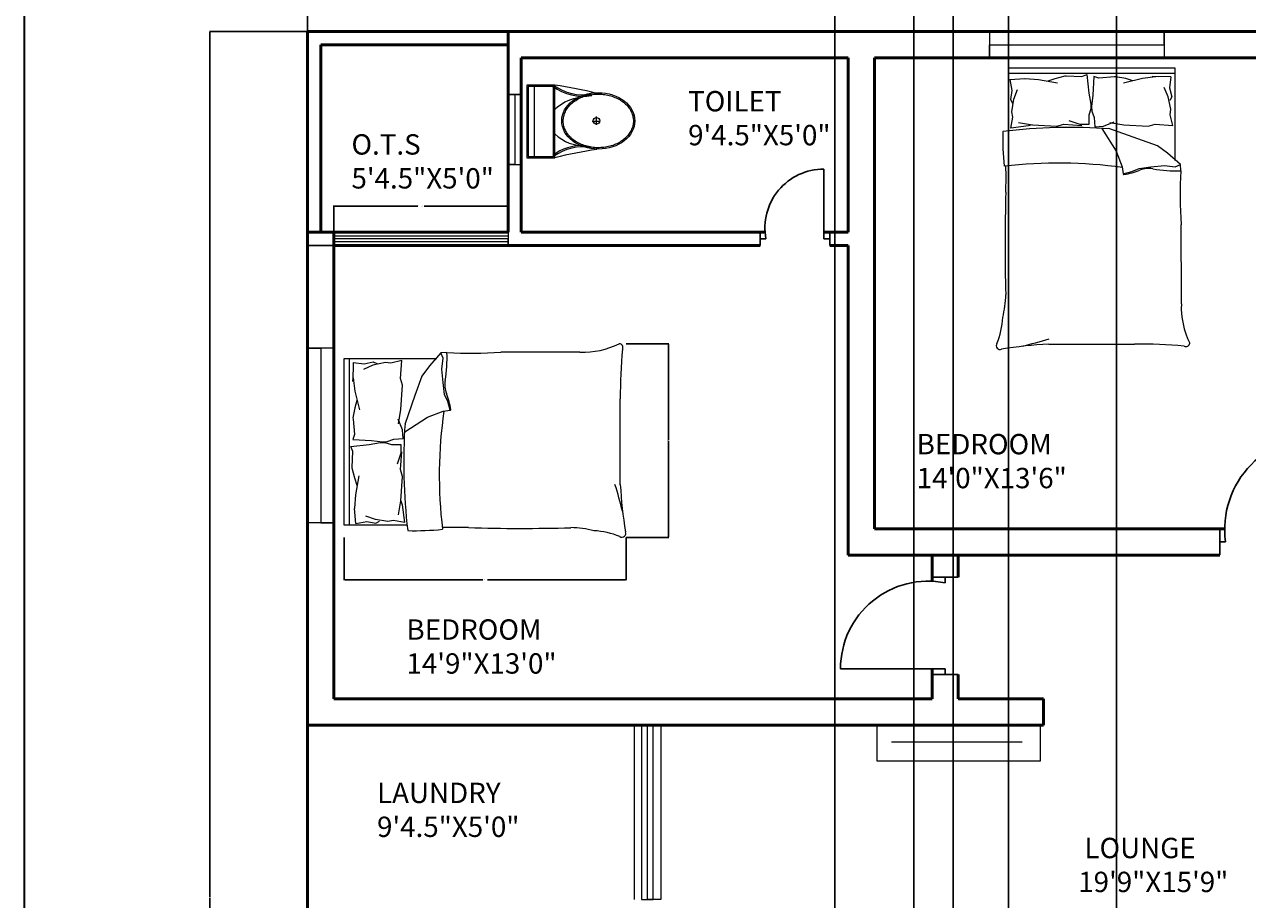
# Model space of a CAD drawing. Units: inches. Extents: x 2215 to 3724, y 1009 to 2124.
# Tile 4 of 11: x 2215 to 2636, y 1449 to 1750. Entities that reach past the tile are written whole.
import ezdxf

# ---------------------------------------------------------------- set-up
doc = ezdxf.new("R2010")
doc.units = ezdxf.units.IN
for name, color, linetype, lineweight in [('A-ANNO-DIMS', 2, 'Continuous', 18), ('A-ANNO-TTLB', 7, 'Continuous', 35), ('A-AREA-IDEN', 7, 'Continuous', 18), ('A-DOOR', 3, 'Continuous', 25), ('A-FLOR-FIXT', 9, 'Continuous', 18), ('A-FURN', 8, 'Continuous', 18), ('A-GLAZ', 4, 'Continuous', 18), ('A-WALL', 7, 'Continuous', 50)]:
    doc.layers.add(name, color=color, linetype=linetype, lineweight=lineweight)
doc.styles.get("Standard").update_dxf_attribs({"font": 'arial.ttf'})
doc.dimstyles.get("Standard").update_dxf_attribs({"dimtxt": 0.18, "dimasz": 0.18, "dimexe": 0.18, "dimexo": 0.0625, "dimgap": 0.09, "dimtad": 0, "dimtih": 1, "dimtoh": 1, "dimdec": 4, "dimzin": 0, "dimdsep": 46, "dimtxsty": 'Standard', "dimcen": 0.09, "dimadec": 0, "dimazin": 0, "dimtfac": 1, "dimtdec": 4, "dimtofl": 0, "dimtmove": 0, "dimatfit": 3, "dimfxl": 1, "dimtolj": 1, "dimtzin": 0, "dimarcsym": 0})

# ---------------------------------------------------------------- blocks, each defined once
blk = doc.blocks.new('A$C31115884')
for p, q in [((283.1, 497.7), (223.4, 497.7)), ((257.5, 466.4), (257.5, 523.2)), ((0, 200), (0, 0)), ((520, 200), (0, 200)), ((10, 190), (10, 10)), ((510, 190), (10, 190)), ((510, 10), (510, 190)), ((520, 0), (520, 200)), ((510, 54.5), (0, 54.5)), ((10, 10), (510, 10)), ((0, 0), (520, 0))]:
    blk.add_line(p, q)
blk.add_circle((255.6, 496.4), 23.6)
for centre, radius, start, end in [((2777.7, -204.6), 2807, 165.4549, 171.71327), ((-294.5, 403.3), 364.7, 324.20913, 9.34987), ((-294.5, 403.3), 374.7, 324.20913, 9.34987), ((805.8, 403.3), 364.7, 170.65013, 215.79087), ((3237, 905), 2807, 188.28673, 194.5451), ((383.6, 406.2), 293.5, 190.27735, 224.15636), ((139.5, 406.2), 293.5, 315.84364, 2.65635), ((805.8, 403.3), 374.7, 179.20365, 215.79087)]:
    blk.add_arc(centre, radius, start, end)
blk.add_ellipse((256.2, 509.9), major_axis=(0, -260.7), ratio=0.772727)
blk.add_open_spline([(256.2, 259.2), (263.1, 259.2), (270, 259.7), (287.8, 262.3), (298.7, 265.1), (319.9, 273.1), (330.2, 278.4), (350.1, 291.1), (359.7, 298.7), (377.7, 315.9), (386.2, 325.5), (401.7, 346.6), (408.8, 358.1), (421.3, 382.5), (426.8, 395.5), (435.9, 422.4), (439.5, 436.4), (444.8, 465.1), (446.5, 479.7), (447.9, 509.2), (447.6, 524), (445, 553.3), (442.7, 567.8), (436.3, 596), (432.1, 609.7), (421.9, 636), (416, 648.6), (402.5, 672.1), (395, 683), (378.6, 703), (369.8, 712.1), (351.1, 728), (341.3, 734.8), (320.9, 746.2), (310.4, 750.7), (288.9, 757.3), (278, 759.4), (256, 761), (245, 760.6), (223.1, 757.2), (212.3, 754.3), (191.1, 746.1), (180.8, 740.7), (160.9, 727.8), (151.4, 720.1), (133.5, 702.7), (125.1, 693), (109.6, 671.7), (102.6, 660.2), (90.2, 635.7), (84.9, 622.7), (76, 595.6), (72.4, 581.6), (67.2, 552.9), (65.6, 538.2), (64.4, 508.8), (64.8, 494), (67.5, 464.7), (69.9, 450.2), (76.6, 422), (80.8, 408.3), (91.1, 382.2), (97.2, 369.7), (110.8, 346.3), (118.4, 335.4), (134.8, 315.6), (143.7, 306.7), (162.4, 290.9), (172.3, 284.2), (192.8, 273), (203.3, 268.6), (224.8, 262.2), (235.8, 260.2), (249.9, 259.3), (253, 259.2), (256.2, 259.2)], degree=3, knots=[0, 0, 0, 0, 0.110105, 0.110105, 0.285049, 0.285049, 0.459994, 0.459994, 0.634938, 0.634938, 0.809882, 0.809882, 0.984827, 0.984827, 1.159771, 1.159771, 1.334715, 1.334715, 1.50966, 1.50966, 1.684604, 1.684604, 1.859549, 1.859549, 2.034493, 2.034493, 2.209437, 2.209437, 2.384382, 2.384382, 2.559326, 2.559326, 2.73427, 2.73427, 2.909215, 2.909215, 3.084159, 3.084159, 3.259103, 3.259103, 3.434048, 3.434048, 3.608992, 3.608992, 3.783936, 3.783936, 3.958881, 3.958881, 4.133825, 4.133825, 4.30877, 4.30877, 4.483714, 4.483714, 4.658658, 4.658658, 4.833603, 4.833603, 5.008547, 5.008547, 5.183491, 5.183491, 5.358436, 5.358436, 5.53338, 5.53338, 5.708324, 5.708324, 5.883269, 5.883269, 6.058213, 6.058213, 6.233158, 6.233158, 6.283185, 6.283185, 6.283185, 6.283185])
blk = doc.blocks.new('DOOR-BEDROOM-N')
for p, q in [((37.14, 4.5), (37.14, 40.5)), ((0, 9), (0, 0)), ((39.14, 9), (39.14, 0)), ((0, 0), (0, 4.5)), ((0, 4.5), (2, 4.5)), ((39.14, 4.5), (37.14, 4.5)), ((39.14, 0), (39.14, 4.5))]:
    blk.add_line(p, q)
blk.add_arc((33.66, 8.74), 31.95, 83.7441, 187.635)
blk = doc.blocks.new('DOOR-BATH-NW')
for p, q in [((21.95, 2.25), (21.95, 26.25)), ((0, 4.5), (0, 0)), ((23.95, 4.5), (23.95, 0)), ((0, 0), (0, 2.25)), ((0, 2.25), (2, 2.25)), ((23.95, 2.25), (21.95, 2.25)), ((23.95, 0), (23.95, 2.25))]:
    blk.add_line(p, q)
blk.add_arc((21.95, 5.96), 20.29, 90, 190.5328)
blk = doc.blocks.new('DOOR-BEDROOM-W')
for p, q in [((40.5, 33.52), (31.5, 33.52)), ((31.5, 33.52), (36, 33.52)), ((36, 33.52), (36, 31.52)), ((36, 2), (0, 2)), ((31.5, 0), (40.5, 0)), ((36, 0), (36, 2)), ((40.5, 0), (36, 0))]:
    blk.add_line(p, q)
blk.add_arc((30.1, 2), 30.1, 78.701, 180)
blk = doc.blocks.new('WIN-60-JAMB-A')
for p, q in [((0, 9), (0, 0)), ((60, 4.5), (60, 9)), ((60, 9), (60, 0)), ((0, 0), (0, 4.5)), ((0, 4.5), (60, 4.5))]:
    blk.add_line(p, q)
blk = doc.blocks.new('SCREEN-LAUNDRY')
for p, q in [((0, 0), (0, 60)), ((0, 60), (9, 60)), ((4.37, 60), (2.37, 60)), ((2.37, 60), (2.37, 0)), ((4.37, 0), (4.37, 60)), ((6.37, 0), (6.37, 60)), ((9, 60), (9, 0)), ((2.37, 0), (4.37, 0)), ((9, 0), (4.37, 0)), ((4.37, 0), (6.37, 0))]:
    blk.add_line(p, q)
blk = doc.blocks.new('VENT-24-NW')
for p, q in [((0, 24), (0, 24)), ((0, 24), (4.5, 24)), ((4.5, 24), (0, 24)), ((0, 24), (2.25, 24)), ((2.25, 24), (2.25, 0)), ((2.25, 0), (0, 0)), ((0, 0), (0, 0)), ((0, 0), (4.5, 0))]:
    blk.add_line(p, q)
blk = doc.blocks.new('WIN-OTS-W')
for p, q in [((60, 4.5), (60, 0)), ((0, 2.25), (0, 3.25)), ((0, 3.25), (60, 3.25)), ((60, 2.25), (0, 2.25)), ((60, 1.25), (0, 1.25)), ((60, 3.25), (60, 2.25)), ((60, 0), (60, 2.25)), ((60, 2.25), (60, 1.25))]:
    blk.add_line(p, q)
blk = doc.blocks.new('BED-DOUBLE')
for p, q in [((33.26, 63.38), (29.37, 58.94)), ((35.35, 63.48), (33.26, 63.38, 4.64)), ((34.01, 61.54), (33.26, 63.38)), ((0, 61.46), (31.9, 61.46)), ((0, 4.17), (0, 61.46)), ((1.84, 4.17), (1.84, 61.46)), ((3.07, 60.08), (2.95, 53.6)), ((3.07, 60.08), (6.91, 59.62)), ((9.9, 59.12), (6.69, 57.7)), ((6.91, 59.62), (10, 60.34)), ((14.18, 60.08), (9.9, 59.12)), ((10, 60.34), (11.25, 59.72)), ((16.11, 59.85), (14.18, 60.08)), ((19.87, 60.78), (16.11, 59.85)), ((19.38, 54.63), (19.87, 60.78)), ((29.37, 58.94), (26.77, 55.41)), ((33.63, 57.82), (34.01, 61.54)), ((2.95, 53.6), (3.05, 54.8)), ((3.05, 54.8), (3.68, 50.25)), ((26.77, 55.41), (24.36, 48.73)), ((34.01, 53.18), (33.63, 57.82)), ((20.05, 52.28), (19.38, 54.63)), ((19.54, 43.87), (20.05, 52.28)), ((34.56, 49.1), (34.01, 53.18)), ((3.68, 50.25), (5.3, 43.75)), ((4.4, 47), (3.69, 44.52)), ((24.36, 48.73), (20.84, 38.73)), ((35.68, 46.68), (34.56, 49.1)), ((36.42, 43.71), (35.68, 46.68)), ((95, 18.06), (95, 47.57)), ((3.69, 44.52), (3.04, 41.01)), ((18.74, 39.04), (19.54, 43.87)), ((28.62, 41.3), (34.01, 43.34)), ((34.01, 43.34), (36.42, 43.71)), ((3.04, 41.01), (3.07, 40.62)), ((3.07, 40.62), (3.57, 35.31)), ((20.07, 36.87), (18.53, 40.55)), ((20.84, 36.28), (28.62, 41.3)), ((3.57, 35.31), (2.99, 33.54)), ((14.84, 32.89), (17.04, 33.72)), ((17.04, 33.72), (20.25, 33.92)), ((20.25, 33.92), (20.07, 36.87)), ((2.24, 31.15), (8.66, 31.84)), ((2.94, 29.42), (2.24, 31.15)), ((2.99, 33.54), (9.43, 33.25)), ((8.66, 31.84), (12.47, 32.54)), ((9.43, 33.25), (13.28, 32.79)), ((12.47, 32.54), (14.03, 32.54)), ((13.28, 32.79), (14.84, 32.89)), ((14.03, 32.54), (16.28, 31.84)), ((16.28, 31.84), (19.5, 31.84)), ((19.5, 31.84), (19.5, 28.9)), ((2.76, 24.09), (2.94, 29.42)), ((19.5, 28.9), (18.19, 25.13)), ((19.38, 23.24), (19.87, 29.39)), ((2.76, 23.7), (2.76, 24.09)), ((3.63, 20.24), (2.76, 23.7)), ((3.98, 14.52), (5.19, 21.1)), ((20.05, 20.89), (19.38, 23.24)), ((4.5, 17.81), (3.63, 20.24)), ((19.54, 12.48), (20.05, 20.89)), ((3.63, 9.93), (3.98, 14.52)), ((3.61, 9.81), (3.63, 9.93)), ((4, 4.67), (3.61, 9.81)), ((18.74, 7.65), (19.54, 12.48)), ((19.54, 12.48), (19.92, 11.13)), ((19.92, 11.13), (20.79, 5.02)), ((3.98, 4.67), (7.79, 5.36)), ((10.74, 6.06), (7.44, 7.27)), ((7.79, 5.36), (10.91, 4.84)), ((15.07, 5.36), (10.74, 6.06)), ((10.91, 4.84), (12.12, 5.54)), ((16.98, 5.71), (15.07, 5.36)), ((20.79, 5.02), (16.98, 5.71)), ((21.71, 4.17), (0, 4.17))]:
    blk.add_line(p, q)
for centre, radius, start, end in [((-7.98, 61.53), 43.38, 349.8763, 2.5657), ((43.54, 218.51), 155.25, 266.9791, 273.8365), ((81.31, -5405.34), 5469.02, 90.00217, 90.28689), ((82.32, 91.3), 27.65, 267.4714, 296.4681), ((94.55, 65.23), 1.32, 332.6588, 86.02), ((254.49, 49.34), 159.5, 174.4998, 180.6351), ((42.04, 52.44), 7.46, 168.6608, 203.7384), ((1.78, 37.35), 35.55, 10.6617, 19.8806), ((187.4, 21.29), 154.68, 171.7845, 186.9006), ((36.49, 43.92), 0.221, 250.2464, 1.1377), ((218.25, 25.61), 197.77, 176.0865, 186.7821), ((-28.43, -20.65), 127.63, 13.3832, 17.7053), ((240.77, 25.69), 145.97, 182.9958, 189.4091), ((24.09, 102.1), 99.87, 268.7218, 275.604), ((37.37, -200.58), 203.94, 88.4762, 91.0082), ((60.68, 581.23), 578.22, 268.22771, 271.71854), ((77.34, -32.25), 35.53, 76.0648, 88.9113), ((84.25, -25.97), 28.25, 67.9751, 86.652), ((95.57, 1.3), 1.31, 236.1736, 23.4781)]:
    blk.add_arc(centre, radius, start, end)
blk = doc.blocks.new('*D43')
at = {"layer": 'A-ANNO-DIMS', "color": 0, "lineweight": -2, "transparency": 16777216}
for p, q in [((2321.84, 1678.56), (2321.84, 1687.68)), ((2322.02, 1687.5), (2350.72, 1687.5)), ((2381.66, 1687.5), (2352.96, 1687.5)), ((2381.84, 1678.56), (2381.84, 1687.68))]:
    blk.add_line(p, q, dxfattribs=at)
at = {"layer": 'A-ANNO-DIMS', "color": 0, "transparency": 16777216}
for points in [[(2322.02, 1687.53), (2322.02, 1687.47), (2321.84, 1687.5)], [(2381.66, 1687.53), (2381.66, 1687.47), (2381.84, 1687.5)]]:
    blk.add_solid(points, dxfattribs=at)
at = {"layer": 'Defpoints', "color": 0, "transparency": 16777216}
for p in [(2381.84, 1687.5), (2321.84, 1678.5), (2381.84, 1678.5)]:
    blk.add_point(p, dxfattribs=at)
at = {"layer": 'A-ANNO-DIMS', "color": 0, "transparency": 16777216, "insert": (2351.84, 1687.5), "char_height": 0.18, "attachment_point": 5}
blk.add_mtext('\\A1;WINDOW 60 TYP.', dxfattribs=at)
blk = doc.blocks.new('*D44')
at = {"layer": 'A-ANNO-DIMS', "color": 0, "lineweight": -2, "transparency": 16777216}
for p, q in [((2321.78, 1678.5), (2312.66, 1678.5)), ((2312.84, 1678.32), (2312.84, 1676.43)), ((2312.84, 1674.18), (2312.84, 1676.07)), ((2321.78, 1674), (2312.66, 1674))]:
    blk.add_line(p, q, dxfattribs=at)
at = {"layer": 'A-ANNO-DIMS', "color": 0, "transparency": 16777216}
for points in [[(2312.81, 1678.32), (2312.87, 1678.32), (2312.84, 1678.5)], [(2312.81, 1674.18), (2312.87, 1674.18), (2312.84, 1674)]]:
    blk.add_solid(points, dxfattribs=at)
at = {"layer": 'Defpoints', "color": 0, "transparency": 16777216}
for p in [(2312.84, 1678.5), (2321.84, 1678.5), (2321.84, 1674)]:
    blk.add_point(p, dxfattribs=at)
at = {"layer": 'A-ANNO-DIMS', "color": 0, "transparency": 16777216, "insert": (2312.84, 1676.25), "char_height": 0.18, "attachment_point": 5}
blk.add_mtext('\\A1;5 TYP.', dxfattribs=at)
blk = doc.blocks.new('*D77')
at = {"layer": 'A-ANNO-DIMS', "color": 0, "lineweight": -2, "transparency": 16777216}
for p, q in [((2325.42, 1573.46), (2325.42, 1558.79)), ((2422.42, 1573.46), (2422.42, 1558.79)), ((2325.6, 1558.97), (2373.1, 1558.97)), ((2422.24, 1558.97), (2374.73, 1558.97))]:
    blk.add_line(p, q, dxfattribs=at)
at = {"layer": 'A-ANNO-DIMS', "color": 0, "transparency": 16777216}
for points in [[(2325.6, 1559), (2325.6, 1558.94), (2325.42, 1558.97)], [(2422.24, 1559), (2422.24, 1558.94), (2422.42, 1558.97)]]:
    blk.add_solid(points, dxfattribs=at)
at = {"layer": 'Defpoints', "color": 0, "transparency": 16777216}
for p in [(2325.42, 1573.52), (2422.42, 1573.52), (2422.42, 1558.97)]:
    blk.add_point(p, dxfattribs=at)
at = {"layer": 'A-ANNO-DIMS', "color": 0, "transparency": 16777216, "insert": (2373.92, 1558.97), "char_height": 0.18, "attachment_point": 5}
blk.add_mtext('\\A1;BED 97 TYP.', dxfattribs=at)
blk = doc.blocks.new('*D78')
at = {"layer": 'A-ANNO-DIMS', "color": 0, "lineweight": -2, "transparency": 16777216}
for p, q in [((2422.48, 1640.18), (2437.15, 1640.18)), ((2436.97, 1640), (2436.97, 1607.03)), ((2436.97, 1573.7), (2436.97, 1606.67)), ((2422.48, 1573.52), (2437.15, 1573.52))]:
    blk.add_line(p, q, dxfattribs=at)
at = {"layer": 'A-ANNO-DIMS', "color": 0, "transparency": 16777216}
for points in [[(2436.94, 1640), (2437, 1640), (2436.97, 1640.18)], [(2436.94, 1573.7), (2437, 1573.7), (2436.97, 1573.52)]]:
    blk.add_solid(points, dxfattribs=at)
at = {"layer": 'Defpoints', "color": 0, "transparency": 16777216}
for p in [(2422.42, 1640.18), (2436.97, 1640.18), (2422.42, 1573.52)]:
    blk.add_point(p, dxfattribs=at)
at = {"layer": 'A-ANNO-DIMS', "color": 0, "transparency": 16777216, "insert": (2436.97, 1606.85), "char_height": 0.18, "attachment_point": 5}
blk.add_mtext('\\A1;67 TYP.', dxfattribs=at)
blk = doc.blocks.new('*D87')
at = {"layer": 'A-ANNO-DIMS', "color": 0, "lineweight": -2, "transparency": 16777216}
for p, q in [((2312.84, 1747.56), (2312.84, 1781.28)), ((2313.02, 1781.1), (2591.55, 1781.1)), ((2870.66, 1781.1), (2592.13, 1781.1)), ((2870.84, 1747.56), (2870.84, 1781.28))]:
    blk.add_line(p, q, dxfattribs=at)
at = {"layer": 'A-ANNO-DIMS', "color": 0, "transparency": 16777216}
for points in [[(2313.02, 1781.13), (2313.02, 1781.07), (2312.84, 1781.1)], [(2870.66, 1781.13), (2870.66, 1781.07), (2870.84, 1781.1)]]:
    blk.add_solid(points, dxfattribs=at)
at = {"layer": 'Defpoints', "color": 0, "transparency": 16777216}
for p in [(2870.84, 1781.1), (2312.84, 1747.5), (2870.84, 1747.5)]:
    blk.add_point(p, dxfattribs=at)
at = {"layer": 'A-ANNO-DIMS', "color": 0, "transparency": 16777216, "insert": (2591.84, 1781.1), "char_height": 0.18, "attachment_point": 5}
blk.add_mtext('\\A1;558', dxfattribs=at)
blk = doc.blocks.new('*D88')
at = {"layer": 'A-ANNO-DIMS', "color": 0, "lineweight": -2, "transparency": 16777216}
for p, q in [((2312.78, 1747.5), (2279.06, 1747.5)), ((2279.24, 1747.32), (2279.24, 1449.93)), ((2279.24, 1152.18), (2279.24, 1449.57)), ((2312.78, 1152), (2279.06, 1152))]:
    blk.add_line(p, q, dxfattribs=at)
at = {"layer": 'A-ANNO-DIMS', "color": 0, "transparency": 16777216}
for points in [[(2279.21, 1747.32), (2279.27, 1747.32), (2279.24, 1747.5)], [(2279.21, 1152.18), (2279.27, 1152.18), (2279.24, 1152)]]:
    blk.add_solid(points, dxfattribs=at)
at = {"layer": 'Defpoints', "color": 0, "transparency": 16777216}
for p in [(2279.24, 1747.5), (2312.84, 1747.5), (2312.84, 1152)]:
    blk.add_point(p, dxfattribs=at)
at = {"layer": 'A-ANNO-DIMS', "color": 0, "transparency": 16777216, "insert": (2279.24, 1449.75), "char_height": 0.18, "attachment_point": 5}
blk.add_mtext('\\A1;595.5', dxfattribs=at)
blk = doc.blocks.new('*D104')
at = {"layer": 'A-ANNO-DIMS', "color": 0, "lineweight": -2, "transparency": 16777216}
for p, q in [((2553.99, 1430.08), (2553.99, 1781.28)), ((2554.17, 1781.1), (2572.13, 1781.1)), ((2590.88, 1781.1), (2572.92, 1781.1)), ((2591.06, 1430.08), (2591.06, 1781.28))]:
    blk.add_line(p, q, dxfattribs=at)
at = {"layer": 'A-ANNO-DIMS', "color": 0, "transparency": 16777216}
for points in [[(2554.17, 1781.13), (2554.17, 1781.07), (2553.99, 1781.1)], [(2590.88, 1781.13), (2590.88, 1781.07), (2591.06, 1781.1)]]:
    blk.add_solid(points, dxfattribs=at)
at = {"layer": 'Defpoints', "color": 0, "transparency": 16777216}
for p in [(2591.06, 1781.1), (2553.99, 1430.02), (2591.06, 1430.02)]:
    blk.add_point(p, dxfattribs=at)
at = {"layer": 'A-ANNO-DIMS', "color": 0, "transparency": 16777216, "insert": (2572.53, 1781.1), "char_height": 0.18, "attachment_point": 5}
blk.add_mtext('\\A1;37.07', dxfattribs=at)
blk = doc.blocks.new('*D106')
at = {"layer": 'A-ANNO-DIMS', "color": 0, "lineweight": -2, "transparency": 16777216}
for p, q in [((2494.2, 1391.49), (2494.2, 1781.28)), ((2494.38, 1781.1), (2507.39, 1781.1)), ((2521.19, 1781.1), (2508.18, 1781.1)), ((2521.37, 1401.43), (2521.37, 1781.28))]:
    blk.add_line(p, q, dxfattribs=at)
at = {"layer": 'A-ANNO-DIMS', "color": 0, "transparency": 16777216}
for points in [[(2494.38, 1781.13), (2494.38, 1781.07), (2494.2, 1781.1)], [(2521.19, 1781.13), (2521.19, 1781.07), (2521.37, 1781.1)]]:
    blk.add_solid(points, dxfattribs=at)
at = {"layer": 'Defpoints', "color": 0, "transparency": 16777216}
for p in [(2521.37, 1781.1), (2521.37, 1401.36), (2494.2, 1391.42)]:
    blk.add_point(p, dxfattribs=at)
at = {"layer": 'A-ANNO-DIMS', "color": 0, "transparency": 16777216, "insert": (2507.78, 1781.1), "char_height": 0.18, "attachment_point": 5}
blk.add_mtext('\\A1;27.18', dxfattribs=at)
blk = doc.blocks.new('*D107')
at = {"layer": 'A-ANNO-DIMS', "color": 0, "lineweight": -2, "transparency": 16777216}
for p, q in [((2534.96, 1425.13), (2534.96, 1781.28)), ((2535.14, 1781.1), (2544.02, 1781.1)), ((2553.81, 1781.1), (2544.93, 1781.1)), ((2553.99, 1430.08), (2553.99, 1781.28))]:
    blk.add_line(p, q, dxfattribs=at)
at = {"layer": 'A-ANNO-DIMS', "color": 0, "transparency": 16777216}
for points in [[(2535.14, 1781.13), (2535.14, 1781.07), (2534.96, 1781.1)], [(2553.81, 1781.13), (2553.81, 1781.07), (2553.99, 1781.1)]]:
    blk.add_solid(points, dxfattribs=at)
at = {"layer": 'Defpoints', "color": 0, "transparency": 16777216}
for p in [(2553.99, 1781.1), (2553.99, 1430.02), (2534.96, 1425.07)]:
    blk.add_point(p, dxfattribs=at)
at = {"layer": 'A-ANNO-DIMS', "color": 0, "transparency": 16777216, "insert": (2544.48, 1781.1), "char_height": 0.18, "attachment_point": 5}
blk.add_mtext('\\A1;19.027', dxfattribs=at)

msp = doc.modelspace()

# ---------------------------------------------------------------- linework, layer by layer
at = {"layer": 'A-ANNO-TTLB'}
msp.add_lwpolyline([(2215.4438, 2124.2681), (3723.6589, 2124.2681), (3723.6589, 1008.7935), (2215.4438, 1008.7935)], close=True, dxfattribs=at)
at = {"layer": 'A-FURN'}
msp.add_line((2513.7219, 1503.2622), (2558.6468, 1503.2622), dxfattribs=at)
msp.add_lwpolyline([(2508.799, 1508.9969), (2564.8187, 1508.9969), (2564.8187, 1496.5376), (2508.799, 1496.5376)], close=True, dxfattribs=at)
at = {"layer": 'A-WALL'}
for p, q in [((2312.841, 1747.4969), (2312.841, 1517.9969)), ((2312.841, 1747.4969), (2870.841, 1747.4969)), ((2381.841, 1747.4969), (2381.841, 1678.4969)), ((2317.341, 1678.4969), (2317.341, 1742.9969)), ((2317.341, 1742.9969), (2381.841, 1742.9969)), ((2386.341, 1738.4969), (2386.341, 1678.4969)), ((2386.341, 1738.4969), (2498.841, 1738.4969)), ((2498.841, 1738.4969), (2498.841, 1678.4969)), ((2507.841, 1738.4969), (2507.841, 1576.4969)), ((2507.841, 1738.4969), (2507.841, 1576.4969)), ((2507.841, 1738.4969), (2675.841, 1738.4969)), ((2321.841, 1678.4969), (2312.841, 1678.4969)), ((2317.341, 1678.4969), (2381.841, 1678.4969)), ((2321.841, 1678.4969), (2317.341, 1678.4969)), ((2321.841, 1673.9969), (2321.841, 1678.4969)), ((2386.341, 1678.4969), (2470.1937, 1678.4969)), ((2490.432, 1678.4969), (2498.841, 1678.4969)), ((2321.841, 1673.9969), (2468.483, 1673.9969)), ((2321.841, 1517.9969), (2321.841, 1673.9969)), ((2492.432, 1673.9969), (2498.841, 1673.9969)), ((2498.841, 1673.9969), (2498.841, 1567.4969)), ((2507.841, 1576.4969), (2628.313, 1576.4969)), ((2507.841, 1576.4969), (2628.313, 1576.4969)), ((2507.841, 1576.4969), (2628.313, 1576.4969)), ((2498.841, 1567.4969), (2626.5952, 1567.4969)), ((2527.6623, 1567.4969), (2527.6623, 1558.4648)), ((2536.6623, 1559.9139), (2536.6623, 1567.4969)), ((2527.6623, 1528.3952), (2527.6623, 1517.9969)), ((2536.6623, 1517.9969), (2536.6623, 1526.3952)), ((2312.841, 1517.9969), (2312.841, 1151.9969)), ((2321.841, 1517.9969), (2527.6623, 1517.9969)), ((2527.6623, 1517.9969), (2527.6623, 1517.9969)), ((2536.6623, 1517.9969), (2566.0091, 1517.9969)), ((2566.0091, 1508.9969), (2566.0091, 1517.9969)), ((2566.0091, 1508.9969), (2312.841, 1508.9969))]:
    msp.add_line(p, q, dxfattribs=at)

# ---------------------------------------------------------------- block references
at = {"layer": 'A-DOOR'}
for name, p in [('DOOR-BATH-NW', (2468.483, 1673.997)), ('DOOR-BEDROOM-N', (2626.595, 1567.497)), ('DOOR-BEDROOM-W', (2496.162, 1526.395))]:
    msp.add_blockref(name, p, dxfattribs=at)
at = {"layer": 'A-FLOR-FIXT', "xscale": 0.048164045903398, "yscale": 0.048164045903398, "zscale": 0.048164045903398, "rotation": 270}
msp.add_blockref('A$C31115884', (2388.2777, 1729.1318), dxfattribs=at)
at = {"layer": 'A-FURN', "rotation": 270}
msp.add_blockref('BED-DOUBLE', (2549.7385, 1735.0364), dxfattribs=at)
at = {"layer": 'A-FURN'}
msp.add_blockref('BED-DOUBLE', (2325.417, 1573.627), dxfattribs=at)
at = {"layer": 'A-GLAZ'}
for name, p in [('WIN-60-JAMB-A', (2547.449, 1738.497)), ('VENT-24-NW', (2381.841, 1701.83)), ('WIN-OTS-W', (2321.841, 1673.997)), ('SCREEN-LAUNDRY', (2425.341, 1448.997))]:
    msp.add_blockref(name, p, dxfattribs=at)
at = {"layer": 'A-GLAZ', "rotation": 270.0000000000003}
msp.add_blockref('WIN-60-JAMB-A', (2312.8411, 1638.611), dxfattribs=at)

# ---------------------------------------------------------------- texts
at = {"layer": 'A-AREA-IDEN', "char_height": 7, "attachment_point": 1}
for s, width, insert in [('TOILET\\P9\'4.5"X5\'0"', 88.455817, (2443.7401, 1727.0784)), ('O.T.S\\P5\'4.5"X5\'0"', 114.583542, (2327.9324, 1712.2153)), ('BEDROOM\\P14\'0"X13\'6"', 97.58298, (2522.357, 1609.1273)), ('BEDROOM\\P14\'9"X13\'0"', 88.16566, (2346.8527, 1545.362)), ('LAUNDRY\\P9\'4.5"X5\'0"', 88.609315, (2336.7317, 1489.1897)), (' LOUNGE\\P19\'9"X15\'9"', 94.665098, (2577.9346, 1470.2222))]:
    msp.add_mtext_dynamic_manual_height_columns(s, width=width, gutter_width=12.5, heights=[0], dxfattribs=dict(at, insert=insert))

# ---------------------------------------------------------------- dimensions: what is measured, and where the dimension line sits
at = {"layer": 'A-ANNO-DIMS'}
for base, p1, p2, override, picture, middle in [((2870.841, 1781.0969), (2312.841, 1747.4969), (2870.841, 1747.4969), {"dimdec": 0, "dimlfac": 1, "dimrnd": 0, "dimzin": 0, "dimdsep": 46, "dimlunit": 2}, '*D87', (2591.841, 1781.0969)), ((2521.3728, 1781.0969), (2494.1952, 1391.4229), (2521.3728, 1401.3639), {"dimdec": 2, "dimlfac": 1, "dimrnd": 0, "dimzin": 0, "dimdsep": 46, "dimlunit": 2}, '*D106', (2507.784, 1781.0969)), ((2553.9914, 1781.0969), (2534.9648, 1425.0681), (2553.9914, 1430.018), {"dimdec": 3, "dimlfac": 1, "dimrnd": 0, "dimzin": 0, "dimdsep": 46, "dimlunit": 2}, '*D107', (2544.4781, 1781.0969)), ((2591.0617, 1781.0969), (2553.9914, 1430.018), (2591.0617, 1430.018), {"dimdec": 2, "dimlfac": 1, "dimrnd": 0, "dimzin": 0, "dimdsep": 46, "dimlunit": 2}, '*D104', (2572.5266, 1781.0969))]:
    dim = msp.add_linear_dim(base=base, p1=p1, p2=p2, dimstyle='Standard', override=override, dxfattribs=at)
    dim.commit()
    dim.dimension.update_dxf_attribs({"geometry": picture, "text_midpoint": middle})
dim = msp.add_linear_dim(base=(2279.241, 1747.4969), p1=(2312.841, 1151.9969), p2=(2312.841, 1747.4969), angle=90, dimstyle='Standard', override={"dimdec": 1, "dimlfac": 1, "dimrnd": 0, "dimzin": 0, "dimdsep": 46, "dimlunit": 2}, dxfattribs=at)
dim.commit()
dim.dimension.update_dxf_attribs({"geometry": '*D88', "text_midpoint": (2279.241, 1449.7469)})
for base, p1, p2, text, picture, middle in [((2381.841, 1687.4969), (2321.841, 1678.4969), (2381.841, 1678.4969), 'WINDOW <> TYP.', '*D43', (2351.841, 1687.4969)), ((2422.4152, 1558.9739), (2325.4165, 1573.5237), (2422.4152, 1573.5237), 'BED <> TYP.', '*D77', (2373.9159, 1558.9739))]:
    dim = msp.add_linear_dim(base=base, p1=p1, p2=p2, text=text, dimstyle='Standard', override={"dimdec": 0, "dimlfac": 1, "dimrnd": 0, "dimzin": 0, "dimdsep": 46, "dimlunit": 2}, dxfattribs=at)
    dim.commit()
    dim.dimension.update_dxf_attribs({"geometry": picture, "text_midpoint": middle})
for base, p1, p2, picture, middle in [((2312.8409975177, 1678.4969403012), (2321.8409975177, 1673.9969403012), (2321.8409975177, 1678.4969403012), '*D44', (2312.8409975177, 1676.2469403012)), ((2436.9651, 1640.1753), (2422.4152, 1573.5237), (2422.4152, 1640.1753), '*D78', (2436.9651, 1606.8495))]:
    dim = msp.add_linear_dim(base=base, p1=p1, p2=p2, angle=90, text='<> TYP.', dimstyle='Standard', override={"dimdec": 0, "dimlfac": 1, "dimrnd": 0, "dimzin": 0, "dimdsep": 46, "dimlunit": 2}, dxfattribs=at)
    dim.commit()
    dim.dimension.update_dxf_attribs({"geometry": picture, "text_midpoint": middle})

doc.saveas('drawing.dxf')
